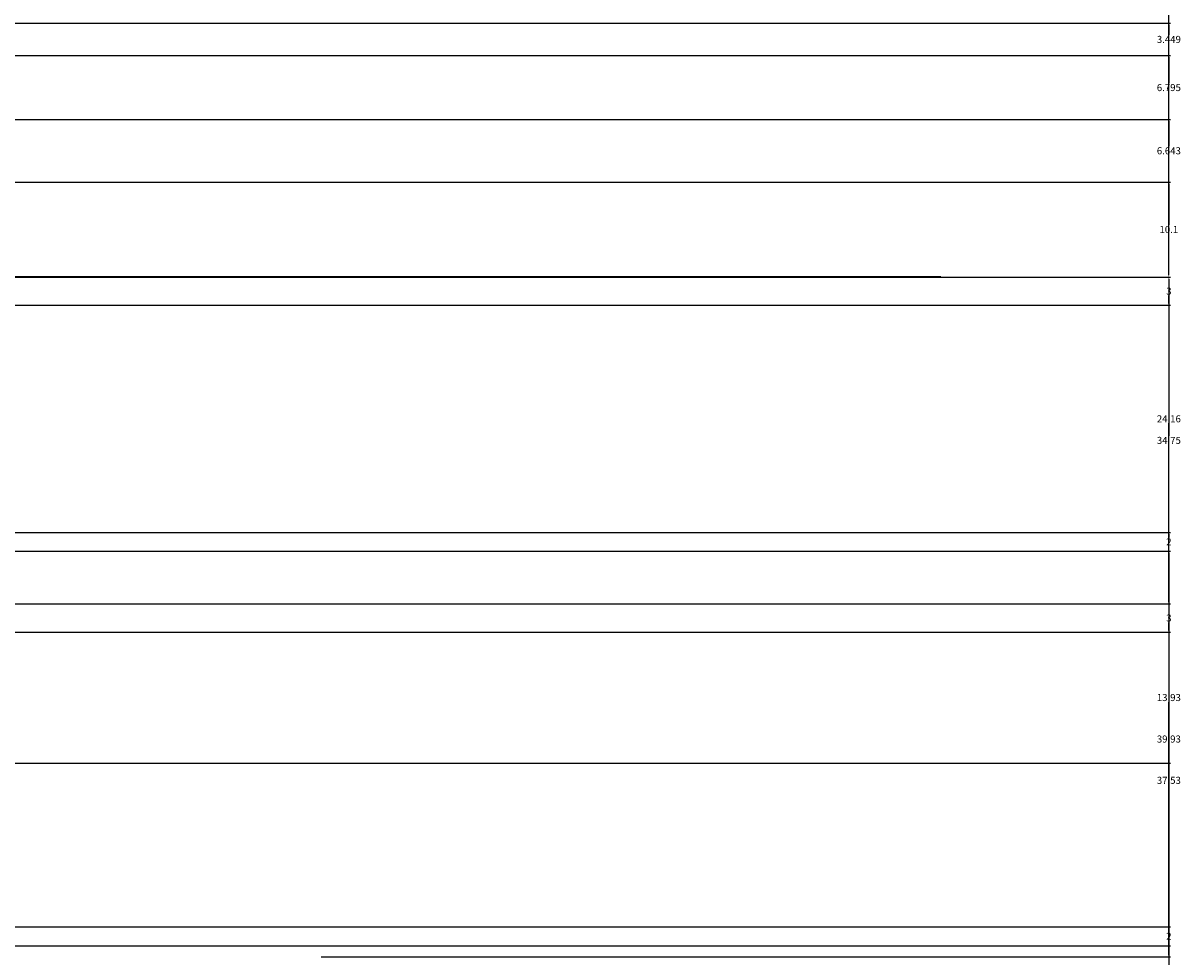
# Model space of a CAD drawing. Units: inches. Extents: x 62 to 566, y 66 to 528.
# Tile 15 of 20: x 443 to 566, y 199 to 298. Entities that reach past the tile are written whole.
import ezdxf

# ---------------------------------------------------------------- set-up
doc = ezdxf.new("R2010")
doc.units = ezdxf.units.IN
doc.header["$MEASUREMENT"] = 0
doc.layers.add('A-ANNO-DIMS', color=2, linetype='Continuous', lineweight=18)
doc.layers.add('A-ELEV', color=7, linetype='Continuous', lineweight=35)
doc.styles.get("Standard").update_dxf_attribs({"font": 'arial.ttf'})
doc.dimstyles.get("Standard").update_dxf_attribs({"dimtxt": 0.75, "dimasz": 0.18, "dimexe": 0.18, "dimexo": 0.0625, "dimgap": 0.09, "dimtad": 0, "dimtih": 1, "dimtoh": 1, "dimdec": 4, "dimzin": 0, "dimdsep": 46, "dimlunit": 4, "dimtxsty": 'Standard', "dimcen": 0.09, "dimadec": 0, "dimazin": 0, "dimtfac": 1, "dimtdec": 4, "dimtofl": 0, "dimtmove": 0, "dimatfit": 3, "dimfxl": 1, "dimtolj": 1, "dimtzin": 0, "dimarcsym": 0})

# ---------------------------------------------------------------- blocks, each defined once
blk = doc.blocks.new('*D20')
at = {"layer": 'A-ANNO-DIMS', "color": 0, "lineweight": -2, "transparency": 16777216}
for p, q in [((474.18, 199.13), (564.47, 199.13)), ((564.29, 198.95), (564.29, 163.22)), ((564.29, 126.55), (564.29, 162.28)), ((474.18, 126.37), (564.47, 126.37))]:
    blk.add_line(p, q, dxfattribs=at)
at = {"layer": 'A-ANNO-DIMS', "color": 0, "transparency": 16777216}
for points in [[(564.26, 198.95), (564.32, 198.95), (564.29, 199.13)], [(564.26, 126.55), (564.32, 126.55), (564.29, 126.37)]]:
    blk.add_solid(points, dxfattribs=at)
at = {"layer": 'Defpoints', "color": 0, "transparency": 16777216}
for p in [(474.12, 199.13), (564.29, 199.13), (474.12, 126.37)]:
    blk.add_point(p, dxfattribs=at)
at = {"layer": 'A-ANNO-DIMS', "color": 0, "transparency": 16777216, "insert": (564.29, 162.75), "char_height": 0.75, "attachment_point": 5}
blk.add_mtext('\\A1;72.76', dxfattribs=at)
blk = doc.blocks.new('*D21')
at = {"layer": 'A-ANNO-DIMS', "color": 0, "lineweight": -2, "transparency": 16777216}
for p, q in [((374.2, 236.66), (564.47, 236.66)), ((564.29, 236.48), (564.29, 218.37)), ((564.29, 199.31), (564.29, 217.42)), ((474.18, 199.13), (564.47, 199.13))]:
    blk.add_line(p, q, dxfattribs=at)
at = {"layer": 'A-ANNO-DIMS', "color": 0, "transparency": 16777216}
for points in [[(564.26, 236.48), (564.32, 236.48), (564.29, 236.66)], [(564.26, 199.31), (564.32, 199.31), (564.29, 199.13)]]:
    blk.add_solid(points, dxfattribs=at)
at = {"layer": 'Defpoints', "color": 0, "transparency": 16777216}
for p in [(374.14, 236.66), (564.29, 236.66), (474.12, 199.13)]:
    blk.add_point(p, dxfattribs=at)
at = {"layer": 'A-ANNO-DIMS', "color": 0, "transparency": 16777216, "insert": (564.29, 217.9), "char_height": 0.75, "attachment_point": 5}
blk.add_mtext('\\A1;37.53', dxfattribs=at)
blk = doc.blocks.new('*D22')
at = {"layer": 'A-ANNO-DIMS', "color": 0, "lineweight": -2, "transparency": 16777216}
for p, q in [((540.1, 271.41), (564.47, 271.41)), ((564.29, 271.23), (564.29, 254.51)), ((564.29, 236.84), (564.29, 253.56)), ((374.2, 236.66), (564.47, 236.66))]:
    blk.add_line(p, q, dxfattribs=at)
at = {"layer": 'A-ANNO-DIMS', "color": 0, "transparency": 16777216}
for points in [[(564.26, 271.23), (564.32, 271.23), (564.29, 271.41)], [(564.26, 236.84), (564.32, 236.84), (564.29, 236.66)]]:
    blk.add_solid(points, dxfattribs=at)
at = {"layer": 'Defpoints', "color": 0, "transparency": 16777216}
for p in [(540.04, 271.41), (564.29, 271.41), (374.14, 236.66)]:
    blk.add_point(p, dxfattribs=at)
at = {"layer": 'A-ANNO-DIMS', "color": 0, "transparency": 16777216, "insert": (564.29, 254.04), "char_height": 0.75, "attachment_point": 5}
blk.add_mtext('\\A1;34.75', dxfattribs=at)
blk = doc.blocks.new('*D23')
at = {"layer": 'A-ANNO-DIMS', "color": 0, "lineweight": -2, "transparency": 16777216}
for p, q in [((374.2, 344.78), (564.47, 344.78)), ((564.29, 344.6), (564.29, 308.57)), ((564.29, 271.59), (564.29, 307.62)), ((540.1, 271.41), (564.47, 271.41))]:
    blk.add_line(p, q, dxfattribs=at)
at = {"layer": 'A-ANNO-DIMS', "color": 0, "transparency": 16777216}
for points in [[(564.26, 344.6), (564.32, 344.6), (564.29, 344.78)], [(564.26, 271.59), (564.32, 271.59), (564.29, 271.41)]]:
    blk.add_solid(points, dxfattribs=at)
at = {"layer": 'Defpoints', "color": 0, "transparency": 16777216}
for p in [(374.14, 344.78), (564.29, 344.78), (540.04, 271.41)]:
    blk.add_point(p, dxfattribs=at)
at = {"layer": 'A-ANNO-DIMS', "color": 0, "transparency": 16777216, "insert": (564.29, 308.1), "char_height": 0.75, "attachment_point": 5}
blk.add_mtext('\\A1;73.37', dxfattribs=at)
blk = doc.blocks.new('*D70')
at = {"layer": 'A-ANNO-DIMS', "color": 0, "lineweight": -2, "transparency": 16777216}
for p, q in [((329.73, 219.73), (564.47, 219.73)), ((564.29, 219.55), (564.29, 175.02)), ((564.29, 129.55), (564.29, 174.08)), ((371.2, 129.37), (564.47, 129.37))]:
    blk.add_line(p, q, dxfattribs=at)
at = {"layer": 'A-ANNO-DIMS', "color": 0, "transparency": 16777216}
for points in [[(564.26, 219.55), (564.32, 219.55), (564.29, 219.73)], [(564.26, 129.55), (564.32, 129.55), (564.29, 129.37)]]:
    blk.add_solid(points, dxfattribs=at)
at = {"layer": 'Defpoints', "color": 0, "transparency": 16777216}
for p in [(329.67, 219.73), (564.29, 219.73), (371.14, 129.37)]:
    blk.add_point(p, dxfattribs=at)
at = {"layer": 'A-ANNO-DIMS', "color": 0, "transparency": 16777216, "insert": (564.29, 174.55), "char_height": 0.75, "attachment_point": 5}
blk.add_mtext('\\A1;90.36', dxfattribs=at)
blk = doc.blocks.new('*D71')
at = {"layer": 'A-ANNO-DIMS', "color": 0, "lineweight": -2, "transparency": 16777216}
for p, q in [((371.2, 233.66), (564.47, 233.66)), ((564.29, 233.48), (564.29, 227.17)), ((564.29, 219.91), (564.29, 226.22)), ((329.73, 219.73), (564.47, 219.73))]:
    blk.add_line(p, q, dxfattribs=at)
at = {"layer": 'A-ANNO-DIMS', "color": 0, "transparency": 16777216}
for points in [[(564.26, 233.48), (564.32, 233.48), (564.29, 233.66)], [(564.26, 219.91), (564.32, 219.91), (564.29, 219.73)]]:
    blk.add_solid(points, dxfattribs=at)
at = {"layer": 'Defpoints', "color": 0, "transparency": 16777216}
for p in [(371.14, 233.66), (564.29, 233.66), (329.67, 219.73)]:
    blk.add_point(p, dxfattribs=at)
at = {"layer": 'A-ANNO-DIMS', "color": 0, "transparency": 16777216, "insert": (564.29, 226.7), "char_height": 0.75, "attachment_point": 5}
blk.add_mtext('\\A1;13.93', dxfattribs=at)
blk = doc.blocks.new('*D72')
at = {"layer": 'A-ANNO-DIMS', "color": 0, "lineweight": -2, "transparency": 16777216}
for p, q in [((374.2, 236.66), (564.47, 236.66)), ((564.29, 236.48), (564.29, 235.63)), ((564.29, 233.84), (564.29, 234.69)), ((371.2, 233.66), (564.47, 233.66))]:
    blk.add_line(p, q, dxfattribs=at)
at = {"layer": 'A-ANNO-DIMS', "color": 0, "transparency": 16777216}
for points in [[(564.26, 236.48), (564.32, 236.48), (564.29, 236.66)], [(564.26, 233.84), (564.32, 233.84), (564.29, 233.66)]]:
    blk.add_solid(points, dxfattribs=at)
at = {"layer": 'Defpoints', "color": 0, "transparency": 16777216}
for p in [(374.14, 236.66), (564.29, 236.66), (371.14, 233.66)]:
    blk.add_point(p, dxfattribs=at)
at = {"layer": 'A-ANNO-DIMS', "color": 0, "transparency": 16777216, "insert": (564.29, 235.16), "char_height": 0.75, "attachment_point": 5}
blk.add_mtext('\\A1;3', dxfattribs=at)
blk = doc.blocks.new('*D88')
at = {"layer": 'A-ANNO-DIMS', "color": 0, "lineweight": -2, "transparency": 16777216}
for p, q in [((433.87, 281.51), (564.47, 281.51)), ((564.29, 281.33), (564.29, 276.94)), ((564.29, 271.59), (564.29, 275.99)), ((439.75, 271.41), (564.47, 271.41))]:
    blk.add_line(p, q, dxfattribs=at)
at = {"layer": 'A-ANNO-DIMS', "color": 0, "transparency": 16777216}
for points in [[(564.26, 281.33), (564.32, 281.33), (564.29, 281.51)], [(564.26, 271.59), (564.32, 271.59), (564.29, 271.41)]]:
    blk.add_solid(points, dxfattribs=at)
at = {"layer": 'Defpoints', "color": 0, "transparency": 16777216}
for p in [(433.81, 281.51), (564.29, 281.51), (439.69, 271.41)]:
    blk.add_point(p, dxfattribs=at)
at = {"layer": 'A-ANNO-DIMS', "color": 0, "transparency": 16777216, "insert": (564.29, 276.46), "char_height": 0.75, "attachment_point": 5}
blk.add_mtext('\\A1;10.1', dxfattribs=at)
blk = doc.blocks.new('*D89')
at = {"layer": 'A-ANNO-DIMS', "color": 0, "lineweight": -2, "transparency": 16777216}
for p, q in [((433.87, 288.16), (564.47, 288.16)), ((564.29, 287.98), (564.29, 285.31)), ((564.29, 281.69), (564.29, 284.36)), ((433.87, 281.51), (564.47, 281.51))]:
    blk.add_line(p, q, dxfattribs=at)
at = {"layer": 'A-ANNO-DIMS', "color": 0, "transparency": 16777216}
for points in [[(564.26, 287.98), (564.32, 287.98), (564.29, 288.16)], [(564.26, 281.69), (564.32, 281.69), (564.29, 281.51)]]:
    blk.add_solid(points, dxfattribs=at)
at = {"layer": 'Defpoints', "color": 0, "transparency": 16777216}
for p in [(433.81, 288.16), (564.29, 288.16), (433.81, 281.51)]:
    blk.add_point(p, dxfattribs=at)
at = {"layer": 'A-ANNO-DIMS', "color": 0, "transparency": 16777216, "insert": (564.29, 284.83), "char_height": 0.75, "attachment_point": 5}
blk.add_mtext('\\A1;6.643', dxfattribs=at)
blk = doc.blocks.new('*D90')
at = {"layer": 'A-ANNO-DIMS', "color": 0, "lineweight": -2, "transparency": 16777216}
for p, q in [((433.87, 294.95), (564.47, 294.95)), ((564.29, 294.77), (564.29, 292.03)), ((564.29, 288.34), (564.29, 291.08)), ((433.87, 288.16), (564.47, 288.16))]:
    blk.add_line(p, q, dxfattribs=at)
at = {"layer": 'A-ANNO-DIMS', "color": 0, "transparency": 16777216}
for points in [[(564.26, 294.77), (564.32, 294.77), (564.29, 294.95)], [(564.26, 288.34), (564.32, 288.34), (564.29, 288.16)]]:
    blk.add_solid(points, dxfattribs=at)
at = {"layer": 'Defpoints', "color": 0, "transparency": 16777216}
for p in [(433.81, 294.95), (564.29, 294.95), (433.81, 288.16)]:
    blk.add_point(p, dxfattribs=at)
at = {"layer": 'A-ANNO-DIMS', "color": 0, "transparency": 16777216, "insert": (564.29, 291.55), "char_height": 0.75, "attachment_point": 5}
blk.add_mtext('\\A1;6.795', dxfattribs=at)
blk = doc.blocks.new('*D91')
at = {"layer": 'A-ANNO-DIMS', "color": 0, "lineweight": -2, "transparency": 16777216}
for p, q in [((433.87, 298.4), (564.47, 298.4)), ((564.29, 298.22), (564.29, 297.15)), ((564.29, 295.13), (564.29, 296.2)), ((433.87, 294.95), (564.47, 294.95))]:
    blk.add_line(p, q, dxfattribs=at)
at = {"layer": 'A-ANNO-DIMS', "color": 0, "transparency": 16777216}
for points in [[(564.26, 298.22), (564.32, 298.22), (564.29, 298.4)], [(564.26, 295.13), (564.32, 295.13), (564.29, 294.95)]]:
    blk.add_solid(points, dxfattribs=at)
at = {"layer": 'Defpoints', "color": 0, "transparency": 16777216}
for p in [(433.81, 298.4), (564.29, 298.4), (433.81, 294.95)]:
    blk.add_point(p, dxfattribs=at)
at = {"layer": 'A-ANNO-DIMS', "color": 0, "transparency": 16777216, "insert": (564.29, 296.67), "char_height": 0.75, "attachment_point": 5}
blk.add_mtext('\\A1;3.449', dxfattribs=at)
blk = doc.blocks.new('*D123')
at = {"layer": 'A-ANNO-DIMS', "color": 0, "lineweight": -2, "transparency": 16777216}
for p, q in [((269.12, 200.32), (564.47, 200.32)), ((564.29, 200.14), (564.29, 182.31)), ((564.29, 163.53), (564.29, 181.37)), ((269.12, 163.35), (564.47, 163.35))]:
    blk.add_line(p, q, dxfattribs=at)
at = {"layer": 'A-ANNO-DIMS', "color": 0, "transparency": 16777216}
for points in [[(564.26, 200.14), (564.32, 200.14), (564.29, 200.32)], [(564.26, 163.53), (564.32, 163.53), (564.29, 163.35)]]:
    blk.add_solid(points, dxfattribs=at)
at = {"layer": 'Defpoints', "color": 0, "transparency": 16777216}
for p in [(269.06, 200.32), (564.29, 200.32), (269.06, 163.35)]:
    blk.add_point(p, dxfattribs=at)
at = {"layer": 'A-ANNO-DIMS', "color": 0, "transparency": 16777216, "insert": (564.29, 181.84), "char_height": 0.75, "attachment_point": 5}
blk.add_mtext('\\A1;36.97', dxfattribs=at)
blk = doc.blocks.new('*D124')
at = {"layer": 'A-ANNO-DIMS', "color": 0, "lineweight": -2, "transparency": 16777216}
for p, q in [((269.12, 202.32), (564.47, 202.32)), ((564.29, 202.14), (564.29, 201.79)), ((564.29, 200.5), (564.29, 200.86)), ((269.12, 200.32), (564.47, 200.32))]:
    blk.add_line(p, q, dxfattribs=at)
at = {"layer": 'A-ANNO-DIMS', "color": 0, "transparency": 16777216}
for points in [[(564.26, 202.14), (564.32, 202.14), (564.29, 202.32)], [(564.26, 200.5), (564.32, 200.5), (564.29, 200.32)]]:
    blk.add_solid(points, dxfattribs=at)
at = {"layer": 'Defpoints', "color": 0, "transparency": 16777216}
for p in [(269.06, 202.32), (564.29, 202.32), (269.06, 200.32)]:
    blk.add_point(p, dxfattribs=at)
at = {"layer": 'A-ANNO-DIMS', "color": 0, "transparency": 16777216, "insert": (564.29, 201.32), "char_height": 0.75, "attachment_point": 5}
blk.add_mtext('\\A1;2', dxfattribs=at)
blk = doc.blocks.new('*D125')
at = {"layer": 'A-ANNO-DIMS', "color": 0, "lineweight": -2, "transparency": 16777216}
for p, q in [((269.12, 242.25), (564.47, 242.25)), ((564.29, 242.07), (564.29, 222.76)), ((564.29, 202.5), (564.29, 221.81)), ((269.12, 202.32), (564.47, 202.32))]:
    blk.add_line(p, q, dxfattribs=at)
at = {"layer": 'A-ANNO-DIMS', "color": 0, "transparency": 16777216}
for points in [[(564.26, 242.07), (564.32, 242.07), (564.29, 242.25)], [(564.26, 202.5), (564.32, 202.5), (564.29, 202.32)]]:
    blk.add_solid(points, dxfattribs=at)
at = {"layer": 'Defpoints', "color": 0, "transparency": 16777216}
for p in [(269.06, 242.25), (564.29, 242.25), (269.06, 202.32)]:
    blk.add_point(p, dxfattribs=at)
at = {"layer": 'A-ANNO-DIMS', "color": 0, "transparency": 16777216, "insert": (564.29, 222.29), "char_height": 0.75, "attachment_point": 5}
blk.add_mtext('\\A1;39.93', dxfattribs=at)
blk = doc.blocks.new('*D126')
at = {"layer": 'A-ANNO-DIMS', "color": 0, "lineweight": -2, "transparency": 16777216}
for p, q in [((269.12, 244.25), (564.47, 244.25)), ((564.29, 244.07), (564.29, 243.72)), ((564.29, 242.43), (564.29, 242.78)), ((269.12, 242.25), (564.47, 242.25))]:
    blk.add_line(p, q, dxfattribs=at)
at = {"layer": 'A-ANNO-DIMS', "color": 0, "transparency": 16777216}
for points in [[(564.26, 244.07), (564.32, 244.07), (564.29, 244.25)], [(564.26, 242.43), (564.32, 242.43), (564.29, 242.25)]]:
    blk.add_solid(points, dxfattribs=at)
at = {"layer": 'Defpoints', "color": 0, "transparency": 16777216}
for p in [(269.06, 244.25), (564.29, 244.25), (269.06, 242.25)]:
    blk.add_point(p, dxfattribs=at)
at = {"layer": 'A-ANNO-DIMS', "color": 0, "transparency": 16777216, "insert": (564.29, 243.25), "char_height": 0.75, "attachment_point": 5}
blk.add_mtext('\\A1;2', dxfattribs=at)
blk = doc.blocks.new('*D127')
at = {"layer": 'A-ANNO-DIMS', "color": 0, "lineweight": -2, "transparency": 16777216}
for p, q in [((269.12, 268.41), (564.47, 268.41)), ((564.29, 268.23), (564.29, 256.8)), ((564.29, 244.43), (564.29, 255.86)), ((269.12, 244.25), (564.47, 244.25))]:
    blk.add_line(p, q, dxfattribs=at)
at = {"layer": 'A-ANNO-DIMS', "color": 0, "transparency": 16777216}
for points in [[(564.26, 268.23), (564.32, 268.23), (564.29, 268.41)], [(564.26, 244.43), (564.32, 244.43), (564.29, 244.25)]]:
    blk.add_solid(points, dxfattribs=at)
at = {"layer": 'Defpoints', "color": 0, "transparency": 16777216}
for p in [(269.06, 268.41), (564.29, 268.41), (269.06, 244.25)]:
    blk.add_point(p, dxfattribs=at)
at = {"layer": 'A-ANNO-DIMS', "color": 0, "transparency": 16777216, "insert": (564.29, 256.33), "char_height": 0.75, "attachment_point": 5}
blk.add_mtext('\\A1;24.16', dxfattribs=at)
blk = doc.blocks.new('*D128')
at = {"layer": 'A-ANNO-DIMS', "color": 0, "lineweight": -2, "transparency": 16777216}
for p, q in [((272.12, 271.41), (564.47, 271.41)), ((564.29, 271.23), (564.29, 270.39)), ((269.12, 268.41), (564.47, 268.41)), ((564.29, 268.59), (564.29, 269.44))]:
    blk.add_line(p, q, dxfattribs=at)
at = {"layer": 'A-ANNO-DIMS', "color": 0, "transparency": 16777216}
for points in [[(564.26, 271.23), (564.32, 271.23), (564.29, 271.41)], [(564.26, 268.59), (564.32, 268.59), (564.29, 268.41)]]:
    blk.add_solid(points, dxfattribs=at)
at = {"layer": 'Defpoints', "color": 0, "transparency": 16777216}
for p in [(272.06, 271.41), (564.29, 271.41), (269.06, 268.41)]:
    blk.add_point(p, dxfattribs=at)
at = {"layer": 'A-ANNO-DIMS', "color": 0, "transparency": 16777216, "insert": (564.29, 269.91), "char_height": 0.75, "attachment_point": 5}
blk.add_mtext('\\A1;3', dxfattribs=at)

msp = doc.modelspace()

# ---------------------------------------------------------------- linework, layer by layer
at = {"layer": 'A-ELEV'}
msp.add_line((217.2752, 271.4128), (540.0368, 271.4128), dxfattribs=at)

# ---------------------------------------------------------------- dimensions: what is measured, and where the dimension line sits
at = {"layer": 'A-ANNO-DIMS'}
for base, p1, p2, override, picture, middle in [((564.2868, 344.7821), (540.0368, 271.4128), (374.1373, 344.7821), {"dimdec": 2, "dimlfac": 1, "dimrnd": 0, "dimzin": 0, "dimdsep": 46, "dimlunit": 2}, '*D23', (564.2868, 308.0974)), ((564.2868, 298.3985), (433.8102, 294.9497), (433.8102, 298.3985), {"dimdec": 3, "dimlfac": 1, "dimrnd": 0, "dimzin": 0, "dimdsep": 46, "dimlunit": 2}, '*D91', (564.2868, 296.6741)), ((564.2868, 294.9497), (433.8102, 288.155), (433.8102, 294.9497), {"dimdec": 3, "dimlfac": 1, "dimrnd": 0, "dimzin": 0, "dimdsep": 46, "dimlunit": 2}, '*D90', (564.2868, 291.5524)), ((564.2868, 288.155), (433.8102, 281.5119), (433.8102, 288.155), {"dimdec": 3, "dimlfac": 1, "dimrnd": 0, "dimzin": 0, "dimdsep": 46, "dimlunit": 2}, '*D89', (564.2868, 284.8335)), ((564.2868, 281.5119), (439.6878, 271.4128), (433.8102, 281.5119), {"dimdec": 1, "dimlfac": 1, "dimrnd": 0, "dimzin": 0, "dimdsep": 46, "dimlunit": 2}, '*D88', (564.2868, 276.4623)), ((564.2868, 271.4128), (269.0586, 268.4128), (272.0586, 271.4128), {"dimdec": 0, "dimlfac": 1, "dimrnd": 0, "dimzin": 0, "dimdsep": 46, "dimlunit": 2}, '*D128', (564.2868, 269.9128)), ((564.2868, 271.4128), (374.1373, 236.6618), (540.0368, 271.4128), {"dimdec": 2, "dimlfac": 1, "dimrnd": 0, "dimzin": 0, "dimdsep": 46, "dimlunit": 2}, '*D22', (564.2868, 254.0373)), ((564.2868, 268.4128), (269.0586, 244.2507), (269.0586, 268.4128), {"dimdec": 2, "dimlfac": 1, "dimrnd": 0, "dimzin": 0, "dimdsep": 46, "dimlunit": 2}, '*D127', (564.2868, 256.3317)), ((564.2868, 244.2507), (269.0586, 242.2507), (269.0586, 244.2507), {"dimdec": 0, "dimlfac": 1, "dimrnd": 0, "dimzin": 0, "dimdsep": 46, "dimlunit": 2}, '*D126', (564.2868, 243.2507)), ((564.2868, 242.2507), (269.0586, 202.3236), (269.0586, 242.2507), {"dimdec": 2, "dimlfac": 1, "dimrnd": 0, "dimzin": 0, "dimdsep": 46, "dimlunit": 2}, '*D125', (564.2868, 222.2872)), ((564.2868, 236.6618), (371.1373, 233.6618), (374.1373, 236.6618), {"dimdec": 0, "dimlfac": 1, "dimrnd": 0, "dimzin": 0, "dimdsep": 46, "dimlunit": 2}, '*D72', (564.2868, 235.1618)), ((564.2868, 236.6618), (474.1214, 199.1332), (374.1373, 236.6618), {"dimdec": 2, "dimlfac": 1, "dimrnd": 0, "dimzin": 0, "dimdsep": 46, "dimlunit": 2}, '*D21', (564.2868, 217.8975)), ((564.2868, 233.6618), (329.6665, 219.7304), (371.1373, 233.6618), {"dimdec": 2, "dimlfac": 1, "dimrnd": 0, "dimzin": 0, "dimdsep": 46, "dimlunit": 2}, '*D71', (564.2868, 226.6961)), ((564.2868, 219.7304), (371.1373, 129.3686), (329.6665, 219.7304), {"dimdec": 2, "dimlfac": 1, "dimrnd": 0, "dimzin": 0, "dimdsep": 46, "dimlunit": 2}, '*D70', (564.2868, 174.5495)), ((564.2868, 202.3236), (269.0586, 200.3236), (269.0586, 202.3236), {"dimdec": 0, "dimlfac": 1, "dimrnd": 0, "dimzin": 0, "dimdsep": 46, "dimlunit": 2}, '*D124', (564.2868, 201.3236)), ((564.2868, 200.3236), (269.0586, 163.3545), (269.0586, 200.3236), {"dimdec": 2, "dimlfac": 1, "dimrnd": 0, "dimzin": 0, "dimdsep": 46, "dimlunit": 2}, '*D123', (564.2868, 181.8391)), ((564.2868, 199.1332), (474.1214, 126.3686), (474.1214, 199.1332), {"dimdec": 2, "dimlfac": 1, "dimrnd": 0, "dimzin": 0, "dimdsep": 46, "dimlunit": 2}, '*D20', (564.2868, 162.7509))]:
    dim = msp.add_linear_dim(base=base, p1=p1, p2=p2, angle=90, dimstyle='Standard', override=override, dxfattribs=at)
    dim.commit()
    dim.dimension.update_dxf_attribs({"geometry": picture, "text_midpoint": middle})

doc.saveas('drawing.dxf')
